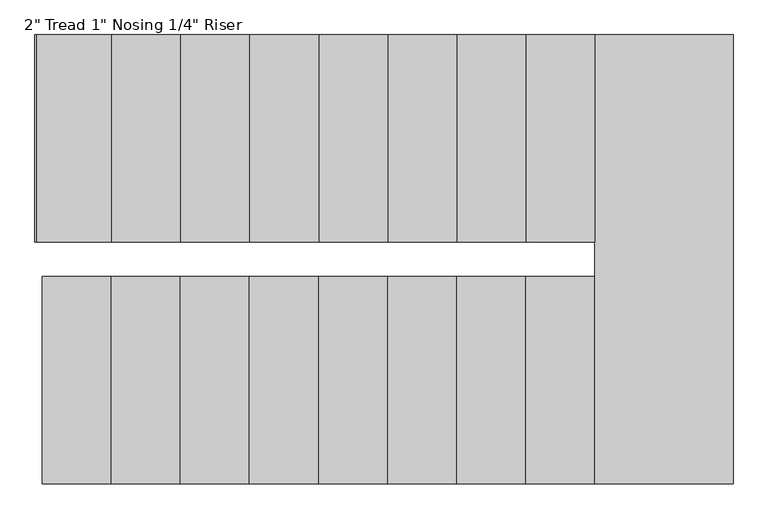
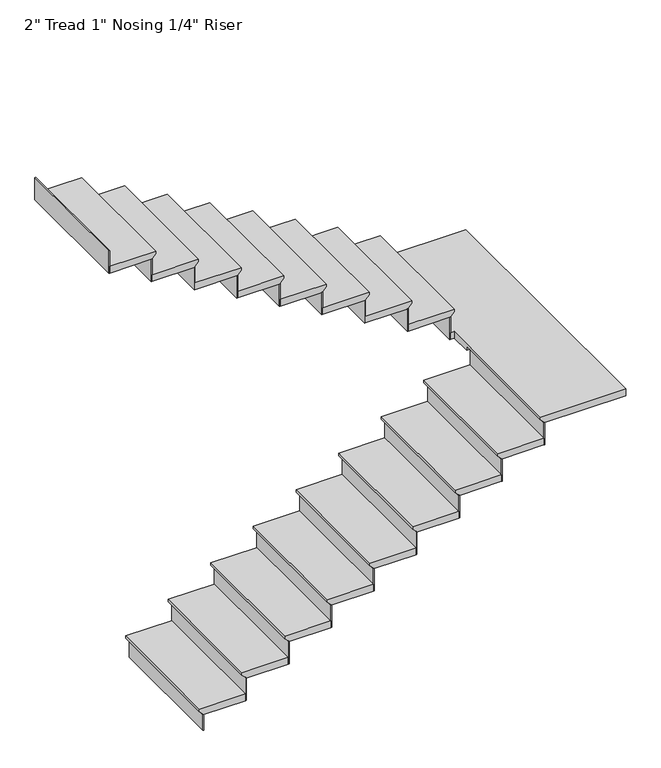
"""IFC4 building model written with IfcOpenShell, lengths in millimetres: stair flight geometry."""

from ifc_helpers import new_model, si_unit, origin, place, context, project, spatial, faceted_brep, source, transform, mapped, element, save


def stair_flight_11d7aa5f(model_context):
    return source(origin(), model_context, "Body", "Brep", [
        faceted_brep([(-1197.97188, -4816.50869, 150.2833333), (-1197.97188, -4816.50869, 169.3333333), (-1197.97188, -3902.10869, 169.3333333), (-1197.97188, -3902.10869, 150.2833333), (-1172.57188, -4816.50869, 124.8833333), (-1172.57188, -3902.10869, 124.8833333), (-867.77188, -4816.50869, 169.3333333), (-867.77188, -3902.10869, 169.3333333), (-1172.57188, -3902.10869, 118.5333333), (-867.77188, -3902.10869, 118.5333333), (-867.77188, -4816.50869, 118.5333333), (-1172.57188, -4816.50869, 118.5333333)], [[[0, 1, 2, 3]], [[4, 0, 3, 5]], [[2, 1, 6, 7]], [[8, 9, 10, 11]], [[2, 7, 9, 8, 5, 3]], [[8, 11, 4, 5]], [[6, 1, 0, 4, 11, 10]], [[7, 6, 10, 9]]]),
        faceted_brep([(-1172.57188, -4816.50869, 118.5333333), (-1172.57188, -4816.50869, 0.0), (-1166.22188, -4816.50869, 0.0), (-1166.22188, -4816.50869, 118.5333333), (-1172.57188, -3902.10869, 118.5333333), (-1166.22188, -3902.10869, 118.5333333), (-1166.22188, -3902.10869, 0.0), (-1172.57188, -3902.10869, 0.0)], [[[0, 1, 2, 3]], [[4, 5, 6, 7]], [[1, 0, 4, 7]], [[2, 1, 7, 6]], [[3, 2, 6, 5]], [[0, 3, 5, 4]]]),
        faceted_brep([(-867.77188, -4816.50869, 287.8666667), (-867.77188, -4816.50869, 118.5333333), (-861.42188, -4816.50869, 118.5333333), (-861.42188, -4816.50869, 287.8666667), (-867.77188, -3902.10869, 287.8666667), (-861.42188, -3902.10869, 287.8666667), (-861.42188, -3902.10869, 118.5333333), (-867.77188, -3902.10869, 118.5333333)], [[[0, 1, 2, 3]], [[4, 5, 6, 7]], [[1, 0, 4, 7]], [[2, 1, 7, 6]], [[3, 2, 6, 5]], [[0, 3, 5, 4]]]),
        faceted_brep([(-893.17188, -3902.10869, 338.6666667), (-893.17188, -4816.50869, 338.6666667), (-562.97188, -4816.50869, 338.6666667), (-562.97188, -3902.10869, 338.6666667), (-867.77188, -3902.10869, 287.8666667), (-562.97188, -3902.10869, 287.8666667), (-562.97188, -4816.50869, 287.8666667), (-867.77188, -4816.50869, 287.8666667), (-867.77188, -3902.10869, 294.2166667), (-893.17188, -3902.10869, 319.6166667), (-867.77188, -4816.50869, 294.2166667), (-893.17188, -4816.50869, 319.6166667)], [[[0, 1, 2, 3]], [[4, 5, 6, 7]], [[0, 3, 5, 4, 8, 9]], [[4, 7, 10, 8]], [[2, 1, 11, 10, 7, 6]], [[3, 2, 6, 5]], [[11, 1, 0, 9]], [[10, 11, 9, 8]]]),
        faceted_brep([(-562.97188, -4816.50869, 457.2), (-562.97188, -4816.50869, 287.8666667), (-556.62188, -4816.50869, 287.8666667), (-556.62188, -4816.50869, 457.2), (-562.97188, -3902.10869, 457.2), (-556.62188, -3902.10869, 457.2), (-556.62188, -3902.10869, 287.8666667), (-562.97188, -3902.10869, 287.8666667)], [[[0, 1, 2, 3]], [[4, 5, 6, 7]], [[1, 0, 4, 7]], [[2, 1, 7, 6]], [[3, 2, 6, 5]], [[0, 3, 5, 4]]]),
        faceted_brep([(-588.37188, -3902.10869, 508.0), (-588.37188, -4816.50869, 508.0), (-258.17188, -4816.50869, 508.0), (-258.17188, -3902.10869, 508.0), (-562.97188, -3902.10869, 457.2), (-258.17188, -3902.10869, 457.2), (-258.17188, -4816.50869, 457.2), (-562.97188, -4816.50869, 457.2), (-562.97188, -3902.10869, 463.55), (-588.37188, -3902.10869, 488.95), (-562.97188, -4816.50869, 463.55), (-588.37188, -4816.50869, 488.95)], [[[0, 1, 2, 3]], [[4, 5, 6, 7]], [[0, 3, 5, 4, 8, 9]], [[4, 7, 10, 8]], [[2, 1, 11, 10, 7, 6]], [[3, 2, 6, 5]], [[11, 1, 0, 9]], [[10, 11, 9, 8]]]),
        faceted_brep([(-258.17188, -4816.50869, 626.5333333), (-258.17188, -4816.50869, 457.2), (-251.82188, -4816.50869, 457.2), (-251.82188, -4816.50869, 626.5333333), (-258.17188, -3902.10869, 626.5333333), (-251.82188, -3902.10869, 626.5333333), (-251.82188, -3902.10869, 457.2), (-258.17188, -3902.10869, 457.2)], [[[0, 1, 2, 3]], [[4, 5, 6, 7]], [[1, 0, 4, 7]], [[2, 1, 7, 6]], [[3, 2, 6, 5]], [[0, 3, 5, 4]]]),
        faceted_brep([(-283.57188, -3902.10869, 677.3333333), (-283.57188, -4816.50869, 677.3333333), (46.62812, -4816.50869, 677.3333333), (46.62812, -3902.10869, 677.3333333), (-258.17188, -3902.10869, 626.5333333), (46.62812, -3902.10869, 626.5333333), (46.62812, -4816.50869, 626.5333333), (-258.17188, -4816.50869, 626.5333333), (-258.17188, -3902.10869, 632.8833333), (-283.57188, -3902.10869, 658.2833333), (-258.17188, -4816.50869, 632.8833333), (-283.57188, -4816.50869, 658.2833333)], [[[0, 1, 2, 3]], [[4, 5, 6, 7]], [[0, 3, 5, 4, 8, 9]], [[4, 7, 10, 8]], [[2, 1, 11, 10, 7, 6]], [[3, 2, 6, 5]], [[11, 1, 0, 9]], [[10, 11, 9, 8]]]),
        faceted_brep([(46.62812, -4816.50869, 795.8666667), (46.62812, -4816.50869, 626.5333333), (52.97812, -4816.50869, 626.5333333), (52.97812, -4816.50869, 795.8666667), (46.62812, -3902.10869, 795.8666667), (52.97812, -3902.10869, 795.8666667), (52.97812, -3902.10869, 626.5333333), (46.62812, -3902.10869, 626.5333333)], [[[0, 1, 2, 3]], [[4, 5, 6, 7]], [[1, 0, 4, 7]], [[2, 1, 7, 6]], [[3, 2, 6, 5]], [[0, 3, 5, 4]]]),
        faceted_brep([(21.22812, -3902.10869, 846.6666667), (21.22812, -4816.50869, 846.6666667), (351.42812, -4816.50869, 846.6666667), (351.42812, -3902.10869, 846.6666667), (46.62812, -3902.10869, 795.8666667), (351.42812, -3902.10869, 795.8666667), (351.42812, -4816.50869, 795.8666667), (46.62812, -4816.50869, 795.8666667), (46.62812, -3902.10869, 802.2166667), (21.22812, -3902.10869, 827.6166667), (46.62812, -4816.50869, 802.2166667), (21.22812, -4816.50869, 827.6166667)], [[[0, 1, 2, 3]], [[4, 5, 6, 7]], [[0, 3, 5, 4, 8, 9]], [[4, 7, 10, 8]], [[2, 1, 11, 10, 7, 6]], [[3, 2, 6, 5]], [[11, 1, 0, 9]], [[10, 11, 9, 8]]]),
        faceted_brep([(351.42812, -4816.50869, 965.2), (351.42812, -4816.50869, 795.8666667), (357.77812, -4816.50869, 795.8666667), (357.77812, -4816.50869, 965.2), (351.42812, -3902.10869, 965.2), (357.77812, -3902.10869, 965.2), (357.77812, -3902.10869, 795.8666667), (351.42812, -3902.10869, 795.8666667)], [[[0, 1, 2, 3]], [[4, 5, 6, 7]], [[1, 0, 4, 7]], [[2, 1, 7, 6]], [[3, 2, 6, 5]], [[0, 3, 5, 4]]]),
        faceted_brep([(326.02812, -3902.10869, 1016.0), (326.02812, -4816.50869, 1016.0), (656.22812, -4816.50869, 1016.0), (656.22812, -3902.10869, 1016.0), (351.42812, -3902.10869, 965.2), (656.22812, -3902.10869, 965.2), (656.22812, -4816.50869, 965.2), (351.42812, -4816.50869, 965.2), (351.42812, -3902.10869, 971.55), (326.02812, -3902.10869, 996.95), (351.42812, -4816.50869, 971.55), (326.02812, -4816.50869, 996.95)], [[[0, 1, 2, 3]], [[4, 5, 6, 7]], [[0, 3, 5, 4, 8, 9]], [[4, 7, 10, 8]], [[2, 1, 11, 10, 7, 6]], [[3, 2, 6, 5]], [[11, 1, 0, 9]], [[10, 11, 9, 8]]]),
        faceted_brep([(656.22812, -4816.50869, 1134.5333333), (656.22812, -4816.50869, 965.2), (662.57812, -4816.50869, 965.2), (662.57812, -4816.50869, 1134.5333333), (656.22812, -3902.10869, 1134.5333333), (662.57812, -3902.10869, 1134.5333333), (662.57812, -3902.10869, 965.2), (656.22812, -3902.10869, 965.2)], [[[0, 1, 2, 3]], [[4, 5, 6, 7]], [[1, 0, 4, 7]], [[2, 1, 7, 6]], [[3, 2, 6, 5]], [[0, 3, 5, 4]]]),
        faceted_brep([(630.82812, -3902.10869, 1185.3333333), (630.82812, -4816.50869, 1185.3333333), (961.02812, -4816.50869, 1185.3333333), (961.02812, -3902.10869, 1185.3333333), (656.22812, -3902.10869, 1134.5333333), (961.02812, -3902.10869, 1134.5333333), (961.02812, -4816.50869, 1134.5333333), (656.22812, -4816.50869, 1134.5333333), (656.22812, -3902.10869, 1140.8833333), (630.82812, -3902.10869, 1166.2833333), (656.22812, -4816.50869, 1140.8833333), (630.82812, -4816.50869, 1166.2833333)], [[[0, 1, 2, 3]], [[4, 5, 6, 7]], [[0, 3, 5, 4, 8, 9]], [[4, 7, 10, 8]], [[2, 1, 11, 10, 7, 6]], [[3, 2, 6, 5]], [[11, 1, 0, 9]], [[10, 11, 9, 8]]]),
        faceted_brep([(961.02812, -4816.50869, 1303.8666667), (961.02812, -4816.50869, 1134.5333333), (967.37812, -4816.50869, 1134.5333333), (967.37812, -4816.50869, 1303.8666667), (961.02812, -3902.10869, 1303.8666667), (967.37812, -3902.10869, 1303.8666667), (967.37812, -3902.10869, 1134.5333333), (961.02812, -3902.10869, 1134.5333333)], [[[0, 1, 2, 3]], [[4, 5, 6, 7]], [[1, 0, 4, 7]], [[2, 1, 7, 6]], [[3, 2, 6, 5]], [[0, 3, 5, 4]]]),
        faceted_brep([(935.62812, -3902.10869, 1354.6666667), (935.62812, -4816.50869, 1354.6666667), (1265.82812, -4816.50869, 1354.6666667), (1265.82812, -3902.10869, 1354.6666667), (961.02812, -3902.10869, 1303.8666667), (1265.82812, -3902.10869, 1303.8666667), (1265.82812, -4816.50869, 1303.8666667), (961.02812, -4816.50869, 1303.8666667), (961.02812, -3902.10869, 1310.2166667), (935.62812, -3902.10869, 1335.6166667), (961.02812, -4816.50869, 1310.2166667), (935.62812, -4816.50869, 1335.6166667)], [[[0, 1, 2, 3]], [[4, 5, 6, 7]], [[0, 3, 5, 4, 8, 9]], [[4, 7, 10, 8]], [[2, 1, 11, 10, 7, 6]], [[3, 2, 6, 5]], [[11, 1, 0, 9]], [[10, 11, 9, 8]]]),
        faceted_brep([(1265.82812, -4816.50869, 1473.2), (1265.82812, -4816.50869, 1303.8666667), (1272.17812, -4816.50869, 1303.8666667), (1272.17812, -4816.50869, 1473.2), (1265.82812, -3902.10869, 1473.2), (1272.17812, -3902.10869, 1473.2), (1272.17812, -3902.10869, 1303.8666667), (1265.82812, -3902.10869, 1303.8666667)], [[[0, 1, 2, 3]], [[4, 5, 6, 7]], [[1, 0, 4, 7]], [[2, 1, 7, 6]], [[3, 2, 6, 5]], [[0, 3, 5, 4]]]),
        faceted_brep([(1215.02812, -3749.70869, 1524.0), (1240.42812, -3749.70869, 1524.0), (1240.42812, -4816.50869, 1524.0), (1850.02812, -4816.50869, 1524.0), (1850.02812, -2835.30869, 1524.0), (1215.02812, -2835.30869, 1524.0), (1240.42812, -3749.70869, 1473.2), (1215.02812, -3749.70869, 1473.2), (1215.02812, -2835.30869, 1473.2), (1850.02812, -2835.30869, 1473.2), (1850.02812, -4816.50869, 1473.2), (1265.82812, -4816.50869, 1473.2), (1265.82812, -3902.10869, 1473.2), (1240.42812, -3902.10869, 1473.2), (1240.42812, -3902.10869, 1504.95), (1240.42812, -4816.50869, 1504.95), (1265.82812, -3902.10869, 1479.55), (1265.82812, -4816.50869, 1479.55)], [[[0, 1, 2, 3, 4, 5]], [[6, 7, 8, 9, 10, 11, 12, 13]], [[1, 0, 7, 6]], [[2, 1, 6, 13, 14, 15]], [[13, 12, 16, 14]], [[12, 11, 17, 16]], [[3, 2, 15, 17, 11, 10]], [[4, 3, 10, 9]], [[5, 4, 9, 8]], [[0, 5, 8, 7]], [[17, 15, 14, 16]]]),
        faceted_brep([(1215.02812, -2835.30869, 1642.5333333), (1215.02812, -2835.30869, 1473.2), (1208.67812, -2835.30869, 1473.2), (1208.67812, -2835.30869, 1642.5333333), (1215.02812, -3749.70869, 1642.5333333), (1208.67812, -3749.70869, 1642.5333333), (1208.67812, -3749.70869, 1473.2), (1215.02812, -3749.70869, 1473.2)], [[[0, 1, 2, 3]], [[4, 5, 6, 7]], [[1, 0, 4, 7]], [[2, 1, 7, 6]], [[3, 2, 6, 5]], [[0, 3, 5, 4]]]),
        faceted_brep([(1240.42812, -3749.70869, 1693.3333333), (1240.42812, -2835.30869, 1693.3333333), (910.22812, -2835.30869, 1693.3333333), (910.22812, -3749.70869, 1693.3333333), (1215.02812, -3749.70869, 1642.5333333), (910.22812, -3749.70869, 1642.5333333), (910.22812, -2835.30869, 1642.5333333), (1215.02812, -2835.30869, 1642.5333333), (1215.02812, -3749.70869, 1648.8833333), (1240.42812, -3749.70869, 1674.2833333), (1215.02812, -2835.30869, 1648.8833333), (1240.42812, -2835.30869, 1674.2833333)], [[[0, 1, 2, 3]], [[4, 5, 6, 7]], [[0, 3, 5, 4, 8, 9]], [[4, 7, 10, 8]], [[2, 1, 11, 10, 7, 6]], [[3, 2, 6, 5]], [[11, 1, 0, 9]], [[10, 11, 9, 8]]]),
        faceted_brep([(910.22812, -2835.30869, 1811.8666667), (910.22812, -2835.30869, 1642.5333333), (903.87812, -2835.30869, 1642.5333333), (903.87812, -2835.30869, 1811.8666667), (910.22812, -3749.70869, 1811.8666667), (903.87812, -3749.70869, 1811.8666667), (903.87812, -3749.70869, 1642.5333333), (910.22812, -3749.70869, 1642.5333333)], [[[0, 1, 2, 3]], [[4, 5, 6, 7]], [[1, 0, 4, 7]], [[2, 1, 7, 6]], [[3, 2, 6, 5]], [[0, 3, 5, 4]]]),
        faceted_brep([(935.62812, -3749.70869, 1862.6666667), (935.62812, -2835.30869, 1862.6666667), (605.42812, -2835.30869, 1862.6666667), (605.42812, -3749.70869, 1862.6666667), (910.22812, -3749.70869, 1811.8666667), (605.42812, -3749.70869, 1811.8666667), (605.42812, -2835.30869, 1811.8666667), (910.22812, -2835.30869, 1811.8666667), (910.22812, -3749.70869, 1818.2166667), (935.62812, -3749.70869, 1843.6166667), (910.22812, -2835.30869, 1818.2166667), (935.62812, -2835.30869, 1843.6166667)], [[[0, 1, 2, 3]], [[4, 5, 6, 7]], [[0, 3, 5, 4, 8, 9]], [[4, 7, 10, 8]], [[2, 1, 11, 10, 7, 6]], [[3, 2, 6, 5]], [[11, 1, 0, 9]], [[10, 11, 9, 8]]]),
        faceted_brep([(605.42812, -2835.30869, 1981.2), (605.42812, -2835.30869, 1811.8666667), (599.07812, -2835.30869, 1811.8666667), (599.07812, -2835.30869, 1981.2), (605.42812, -3749.70869, 1981.2), (599.07812, -3749.70869, 1981.2), (599.07812, -3749.70869, 1811.8666667), (605.42812, -3749.70869, 1811.8666667)], [[[0, 1, 2, 3]], [[4, 5, 6, 7]], [[1, 0, 4, 7]], [[2, 1, 7, 6]], [[3, 2, 6, 5]], [[0, 3, 5, 4]]]),
        faceted_brep([(630.82812, -3749.70869, 2032.0), (630.82812, -2835.30869, 2032.0), (300.62812, -2835.30869, 2032.0), (300.62812, -3749.70869, 2032.0), (605.42812, -3749.70869, 1981.2), (300.62812, -3749.70869, 1981.2), (300.62812, -2835.30869, 1981.2), (605.42812, -2835.30869, 1981.2), (605.42812, -3749.70869, 1987.55), (630.82812, -3749.70869, 2012.95), (605.42812, -2835.30869, 1987.55), (630.82812, -2835.30869, 2012.95)], [[[0, 1, 2, 3]], [[4, 5, 6, 7]], [[0, 3, 5, 4, 8, 9]], [[4, 7, 10, 8]], [[2, 1, 11, 10, 7, 6]], [[3, 2, 6, 5]], [[11, 1, 0, 9]], [[10, 11, 9, 8]]]),
        faceted_brep([(300.62812, -2835.30869, 2150.5333333), (300.62812, -2835.30869, 1981.2), (294.27812, -2835.30869, 1981.2), (294.27812, -2835.30869, 2150.5333333), (300.62812, -3749.70869, 2150.5333333), (294.27812, -3749.70869, 2150.5333333), (294.27812, -3749.70869, 1981.2), (300.62812, -3749.70869, 1981.2)], [[[0, 1, 2, 3]], [[4, 5, 6, 7]], [[1, 0, 4, 7]], [[2, 1, 7, 6]], [[3, 2, 6, 5]], [[0, 3, 5, 4]]]),
        faceted_brep([(326.02812, -3749.70869, 2201.3333333), (326.02812, -2835.30869, 2201.3333333), (-4.17188, -2835.30869, 2201.3333333), (-4.17188, -3749.70869, 2201.3333333), (300.62812, -3749.70869, 2150.5333333), (-4.17188, -3749.70869, 2150.5333333), (-4.17188, -2835.30869, 2150.5333333), (300.62812, -2835.30869, 2150.5333333), (300.62812, -3749.70869, 2156.8833333), (326.02812, -3749.70869, 2182.2833333), (300.62812, -2835.30869, 2156.8833333), (326.02812, -2835.30869, 2182.2833333)], [[[0, 1, 2, 3]], [[4, 5, 6, 7]], [[0, 3, 5, 4, 8, 9]], [[4, 7, 10, 8]], [[2, 1, 11, 10, 7, 6]], [[3, 2, 6, 5]], [[11, 1, 0, 9]], [[10, 11, 9, 8]]]),
        faceted_brep([(-4.17188, -2835.30869, 2319.8666667), (-4.17188, -2835.30869, 2150.5333333), (-10.52188, -2835.30869, 2150.5333333), (-10.52188, -2835.30869, 2319.8666667), (-4.17188, -3749.70869, 2319.8666667), (-10.52188, -3749.70869, 2319.8666667), (-10.52188, -3749.70869, 2150.5333333), (-4.17188, -3749.70869, 2150.5333333)], [[[0, 1, 2, 3]], [[4, 5, 6, 7]], [[1, 0, 4, 7]], [[2, 1, 7, 6]], [[3, 2, 6, 5]], [[0, 3, 5, 4]]]),
        faceted_brep([(21.22812, -3749.70869, 2370.6666667), (21.22812, -2835.30869, 2370.6666667), (-308.97188, -2835.30869, 2370.6666667), (-308.97188, -3749.70869, 2370.6666667), (-4.17188, -3749.70869, 2319.8666667), (-308.97188, -3749.70869, 2319.8666667), (-308.97188, -2835.30869, 2319.8666667), (-4.17188, -2835.30869, 2319.8666667), (-4.17188, -3749.70869, 2326.2166667), (21.22812, -3749.70869, 2351.6166667), (-4.17188, -2835.30869, 2326.2166667), (21.22812, -2835.30869, 2351.6166667)], [[[0, 1, 2, 3]], [[4, 5, 6, 7]], [[0, 3, 5, 4, 8, 9]], [[4, 7, 10, 8]], [[2, 1, 11, 10, 7, 6]], [[3, 2, 6, 5]], [[11, 1, 0, 9]], [[10, 11, 9, 8]]]),
        faceted_brep([(-308.97188, -2835.30869, 2489.2), (-308.97188, -2835.30869, 2319.8666667), (-315.32188, -2835.30869, 2319.8666667), (-315.32188, -2835.30869, 2489.2), (-308.97188, -3749.70869, 2489.2), (-315.32188, -3749.70869, 2489.2), (-315.32188, -3749.70869, 2319.8666667), (-308.97188, -3749.70869, 2319.8666667)], [[[0, 1, 2, 3]], [[4, 5, 6, 7]], [[1, 0, 4, 7]], [[2, 1, 7, 6]], [[3, 2, 6, 5]], [[0, 3, 5, 4]]]),
        faceted_brep([(-283.57188, -3749.70869, 2540.0), (-283.57188, -2835.30869, 2540.0), (-613.77188, -2835.30869, 2540.0), (-613.77188, -3749.70869, 2540.0), (-308.97188, -3749.70869, 2489.2), (-613.77188, -3749.70869, 2489.2), (-613.77188, -2835.30869, 2489.2), (-308.97188, -2835.30869, 2489.2), (-308.97188, -3749.70869, 2495.55), (-283.57188, -3749.70869, 2520.95), (-308.97188, -2835.30869, 2495.55), (-283.57188, -2835.30869, 2520.95)], [[[0, 1, 2, 3]], [[4, 5, 6, 7]], [[0, 3, 5, 4, 8, 9]], [[4, 7, 10, 8]], [[2, 1, 11, 10, 7, 6]], [[3, 2, 6, 5]], [[11, 1, 0, 9]], [[10, 11, 9, 8]]]),
        faceted_brep([(-613.77188, -2835.30869, 2658.5333333), (-613.77188, -2835.30869, 2489.2), (-620.12188, -2835.30869, 2489.2), (-620.12188, -2835.30869, 2658.5333333), (-613.77188, -3749.70869, 2658.5333333), (-620.12188, -3749.70869, 2658.5333333), (-620.12188, -3749.70869, 2489.2), (-613.77188, -3749.70869, 2489.2)], [[[0, 1, 2, 3]], [[4, 5, 6, 7]], [[1, 0, 4, 7]], [[2, 1, 7, 6]], [[3, 2, 6, 5]], [[0, 3, 5, 4]]]),
        faceted_brep([(-588.37188, -3749.70869, 2709.3333333), (-588.37188, -2835.30869, 2709.3333333), (-918.57188, -2835.30869, 2709.3333333), (-918.57188, -3749.70869, 2709.3333333), (-613.77188, -3749.70869, 2658.5333333), (-918.57188, -3749.70869, 2658.5333333), (-918.57188, -2835.30869, 2658.5333333), (-613.77188, -2835.30869, 2658.5333333), (-613.77188, -3749.70869, 2664.8833333), (-588.37188, -3749.70869, 2690.2833333), (-613.77188, -2835.30869, 2664.8833333), (-588.37188, -2835.30869, 2690.2833333)], [[[0, 1, 2, 3]], [[4, 5, 6, 7]], [[0, 3, 5, 4, 8, 9]], [[4, 7, 10, 8]], [[2, 1, 11, 10, 7, 6]], [[3, 2, 6, 5]], [[11, 1, 0, 9]], [[10, 11, 9, 8]]]),
        faceted_brep([(-918.57188, -2835.30869, 2827.8666667), (-918.57188, -2835.30869, 2658.5333333), (-924.92188, -2835.30869, 2658.5333333), (-924.92188, -2835.30869, 2827.8666667), (-918.57188, -3749.70869, 2827.8666667), (-924.92188, -3749.70869, 2827.8666667), (-924.92188, -3749.70869, 2658.5333333), (-918.57188, -3749.70869, 2658.5333333)], [[[0, 1, 2, 3]], [[4, 5, 6, 7]], [[1, 0, 4, 7]], [[2, 1, 7, 6]], [[3, 2, 6, 5]], [[0, 3, 5, 4]]]),
        faceted_brep([(-1223.37188, -2835.30869, 2997.2), (-1223.37188, -2835.30869, 2827.8666667), (-1229.72188, -2835.30869, 2827.8666667), (-1229.72188, -2835.30869, 2997.2), (-1223.37188, -3749.70869, 2997.2), (-1229.72188, -3749.70869, 2997.2), (-1229.72188, -3749.70869, 2827.8666667), (-1223.37188, -3749.70869, 2827.8666667)], [[[0, 1, 2, 3]], [[4, 5, 6, 7]], [[1, 0, 4, 7]], [[2, 1, 7, 6]], [[3, 2, 6, 5]], [[0, 3, 5, 4]]]),
        faceted_brep([(-893.17188, -3749.70869, 2878.6666667), (-893.17188, -2835.30869, 2878.6666667), (-1223.37188, -2835.30869, 2878.6666667), (-1223.37188, -3749.70869, 2878.6666667), (-918.57188, -3749.70869, 2827.8666667), (-1223.37188, -3749.70869, 2827.8666667), (-1223.37188, -2835.30869, 2827.8666667), (-918.57188, -2835.30869, 2827.8666667), (-918.57188, -3749.70869, 2834.2166667), (-893.17188, -3749.70869, 2859.6166667), (-918.57188, -2835.30869, 2834.2166667), (-893.17188, -2835.30869, 2859.6166667)], [[[0, 1, 2, 3]], [[4, 5, 6, 7]], [[0, 3, 5, 4, 8, 9]], [[4, 7, 10, 8]], [[2, 1, 11, 10, 7, 6]], [[3, 2, 6, 5]], [[11, 1, 0, 9]], [[10, 11, 9, 8]]]),
    ])


if __name__ == "__main__":
    model = new_model("IFC4")
    model_context = context("Model", 3, world=origin())
    ifc_project = project(units=[si_unit("LENGTHUNIT", "METRE", prefix="MILLI")], contexts=[model_context])
    site = spatial("IfcSite", under=ifc_project)
    building = spatial("IfcBuilding", under=site)
    placement = place(None, origin())
    stair_flight_shape = stair_flight_11d7aa5f(model_context)
    element("IfcStairFlight", 1, ObjectType="2\" Tread 1\" Nosing 1/4\" Riser", at=placement, inside=building, context=model_context, shape_type="MappedRepresentation", body=[
        mapped(stair_flight_shape, transform((0.0, 0.0, 0.0), x_axis=(1.0, 0.0, 0.0), y_axis=(0.0, 1.0, 0.0), z_axis=(0.0, 0.0, 1.0))),
    ])
    save(model, "model.ifc")
